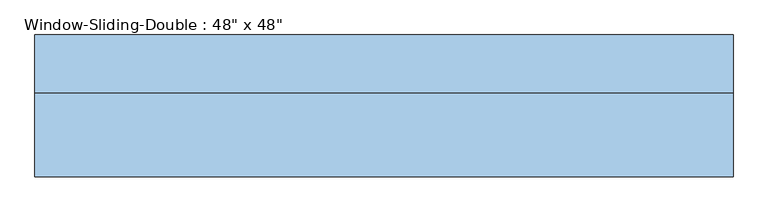
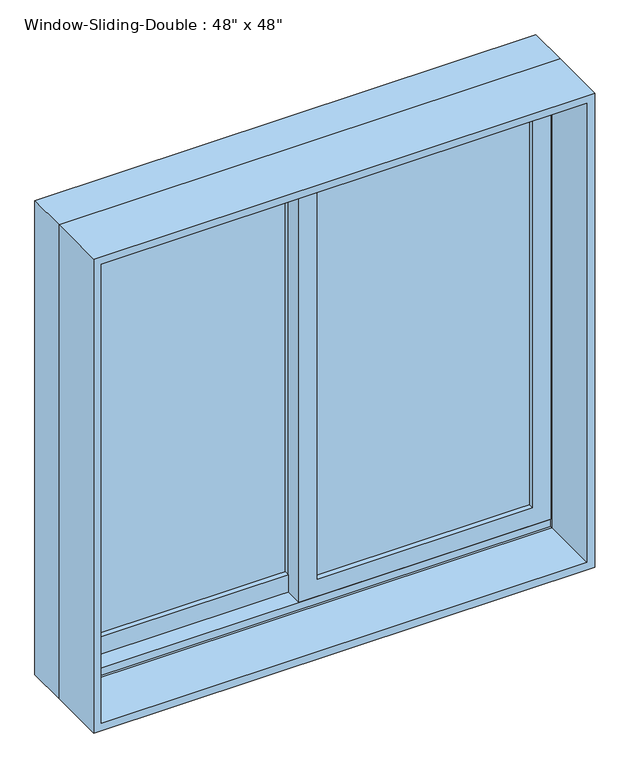
"""IFC4 building model written with IfcOpenShell, lengths in millimetres: window geometry."""

from ifc_helpers import new_model, si_unit, frame, origin, place, context, project, spatial, polyline, outline, extrude, faceted_brep, source, transform, mapped, element, save


def window_5af5dca6(model_context):
    return source(origin(), model_context, "Body", "SolidModel", [
        extrude(outline(polyline([(952.5, 590.55), (2114.55, 590.55), (2114.55, -22.225), (952.5, -22.225), (952.5, 590.55)]), holes=[polyline([(996.95, 22.225), (2070.1, 22.225), (2070.1, 546.1), (996.95, 546.1), (996.95, 22.225)])]), frame((0.0, 34.29, 0.0), z_axis=(0.0, 1.0, 0.0), x_axis=(0.0, 0.0, 1.0)), (0.0, 0.0, 1.0), 44.45),
        extrude(outline(polyline([(933.45, -590.55), (933.45, 22.225), (2114.55, 22.225), (2114.55, -590.55), (933.45, -590.55)]), holes=[polyline([(2070.1, -22.225), (996.95, -22.225), (996.95, -546.1), (2070.1, -546.1), (2070.1, -22.225)])]), frame((0.0, 78.74, 0.0), z_axis=(0.0, 1.0, 0.0), x_axis=(0.0, 0.0, 1.0)), (0.0, 0.0, 1.0), 44.45),
        extrude(outline(polyline([(-22.225, 110.49), (-22.225, 104.14), (-546.1, 104.14), (-546.1, 110.49), (-22.225, 110.49)])), frame((0.0, 0.0, 996.95), z_axis=(0.0, 0.0, 1.0), x_axis=(1.0, 0.0, 0.0)), (0.0, 0.0, 1.0), 1073.15),
        extrude(outline(polyline([(-22.225, 97.79), (-22.225, 91.44), (-546.1, 91.44), (-546.1, 97.79), (-22.225, 97.79)])), frame((0.0, 0.0, 996.95), z_axis=(0.0, 0.0, 1.0), x_axis=(1.0, 0.0, 0.0)), (0.0, 0.0, 1.0), 1073.15),
        extrude(outline(polyline([(546.1, 66.04), (546.1, 59.69), (22.225, 59.69), (22.225, 66.04), (546.1, 66.04)])), frame((0.0, 0.0, 996.95), z_axis=(0.0, 0.0, 1.0), x_axis=(1.0, 0.0, 0.0)), (0.0, 0.0, 1.0), 1073.15),
        extrude(outline(polyline([(546.1, 53.34), (546.1, 46.99), (22.225, 46.99), (22.225, 53.34), (546.1, 53.34)])), frame((0.0, 0.0, 996.95), z_axis=(0.0, 0.0, 1.0), x_axis=(1.0, 0.0, 0.0)), (0.0, 0.0, 1.0), 1073.15),
        extrude(outline(polyline([(2133.6, -609.6), (914.4, -609.6), (914.4, 609.6), (2133.6, 609.6), (2133.6, -609.6)]), holes=[polyline([(2114.55, 590.55), (933.45, 590.55), (933.45, -590.55), (2114.55, -590.55), (2114.55, 590.55)])]), frame((0.0, -118.11, 0.0), z_axis=(0.0, 1.0, 0.0), x_axis=(0.0, 0.0, 1.0)), (0.0, 0.0, 1.0), 146.05),
        faceted_brep([(-609.6, 27.94, 914.4), (-609.6, 129.54, 914.4), (609.6, 129.54, 914.4), (609.6, 27.94, 914.4), (-568.6778905, 129.54, 2092.6778905), (-568.6778905, 123.19, 2092.6778905), (-568.6778905, 123.19, 933.45), (-568.6778905, 129.54, 933.45), (568.6778905, 123.19, 2092.6778905), (568.6778905, 123.19, 933.45), (590.55, 123.19, 933.45), (590.55, 123.19, 2114.55), (-590.55, 123.19, 2114.55), (-590.55, 123.19, 933.45), (-590.55, 27.94, 2114.55), (-590.55, 27.94, 933.45), (-590.55, 34.29, 933.45), (-590.55, 34.29, 952.5), (-590.55, 78.74, 952.5), (-590.55, 78.74, 933.45), (609.6, 27.94, 2133.6), (-609.6, 27.94, 2133.6), (590.55, 27.94, 2114.55), (590.55, 27.94, 933.45), (-609.6, 129.54, 2133.6), (609.6, 129.54, 2133.6), (568.6778905, 129.54, 933.45), (568.6778905, 129.54, 2092.6778905), (590.55, 78.74, 933.45), (590.55, 78.74, 952.5), (590.55, 34.29, 952.5), (590.55, 34.29, 933.45)], [[[0, 1, 2, 3]], [[4, 5, 6, 7]], [[5, 8, 9, 10, 11, 12, 13, 6]], [[12, 14, 15, 16, 17, 18, 19, 13]], [[0, 3, 20, 21], [22, 23, 15, 14]], [[24, 1, 0, 21]], [[2, 1, 24, 25], [4, 7, 26, 27]], [[5, 4, 27, 8]], [[12, 11, 22, 14]], [[21, 20, 25, 24]], [[8, 27, 26, 9]], [[22, 11, 10, 28, 29, 30, 31, 23]], [[20, 3, 2, 25]], [[26, 7, 6, 13, 19, 28, 10, 9]], [[28, 19, 18, 29]], [[29, 18, 17, 30]], [[30, 17, 16, 31]], [[15, 23, 31, 16]]]),
    ])


if __name__ == "__main__":
    model = new_model("IFC4")
    model_context = context("Model", 3, world=origin())
    ifc_project = project(units=[si_unit("LENGTHUNIT", "METRE", prefix="MILLI")], contexts=[model_context])
    site = spatial("IfcSite", under=ifc_project)
    building = spatial("IfcBuilding", under=site)
    placement = place(None, origin())
    window_shape = window_5af5dca6(model_context)
    element("IfcWindow", 1, ObjectType="Window-Sliding-Double : 48\" x 48\"", at=placement, inside=building, context=model_context, shape_type="MappedRepresentation", body=[
        mapped(window_shape, transform((0.0, 0.0, 0.0), x_axis=(1.0, 0.0, 0.0), y_axis=(0.0, 1.0, 0.0), z_axis=(0.0, 0.0, 1.0))),
    ])
    save(model, "model.ifc")

# Revit data of these elements
# Type "Window-Sliding-Double : 48\" x 48\""
#   Type Mark = "22"
#   Fire Rating = "0.5h"
#   Assembly Code = "B2020100"
#   Analytic Construction = "Double glazing - domestic"
#   Window Inset [instance default] = 0' - 0"
#   Wall Thickness [instance default] = 0' - 6"
#   Visual Light Transmittance = 0.81
#   Thermal Resistance (R) = 1.8146 (h·ft²·°F)/BTU
#   Solar Heat Gain Coefficient = 0.76
#   Muntin Width = 1' - 8 5/8"
#   Muntin Height = 3' - 6 1/4"
#   Interior Wall Closure [instance default] = 0' - 2 3/4"
#   Heat Transfer Coefficient (U) = 0.5511 BTU/(h·ft²·°F)
#   Frame Extension [instance default] = 0' - 0 1/4"
#   Exterior Wall Closure [instance default] = 0' - 1 1/4"
#   Rough Width = 4' - 0 1/2"
#   Rough Height = 4' - 0 1/2"
#   Height = 4' - 0"
#   Extension Jamb [instance default] = 0' - 2 3/4"
#   Default Sill Height = 3' - 0"
#   Width = 4' - 0"
#   Interior Trim Visibility [instance default] = yes
#   Indicator Visibility [instance default] = yes
#   Exterior Trim Visibility [instance default] = yes
#   Muntin Visibility = yes
#   Extension Jamb Visibility [instance default] = yes
#   Muntin Pattern = Muntin Pattern_2x2 : Muntin Pattern_2x2
#   Interior Trim Material = Wood - Stained
#   Interior Trim = Trim-Window-Interior-Flat : Picture Frame
#   Interior Frame Material = Wood - Stained
#   Glass Panel Material = Glass
#   Exterior Trim Material = Clad - White
#   Exterior Trim = Trim-Window-Exterior-Flat : with Sill
#   Exterior Frame Material = Clad - White
#   Wall Closure = (empty or 0)
# Element 1 (IfcWindow, "Window-Sliding-Double : 48\" x 48\"")
#   Wall Thickness = 0' - 9"
#   Extension Jamb = 0' - 5 3/4"
#   Materials on its faces: "Wood - Stained", "Glass", "Clad - White"
# Materials
#   "Wood - Stained": class "Wood", colour RGB 224 178 126, transparency 0, Cost = 0
#   "Glass": class "Glass", colour RGB 0 128 192, transparency 0.75, Description = "Soda Lime Glass", Cost = 0
#   "Clad - White": class "Wood", colour RGB 242 242 238, transparency 0, Cost = 0
